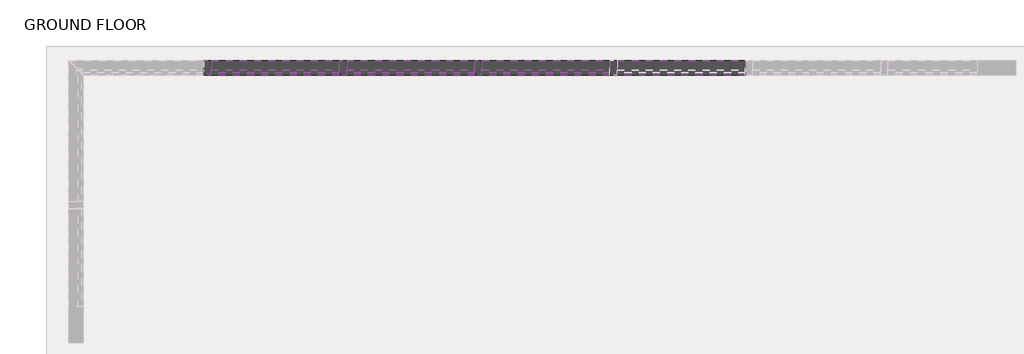
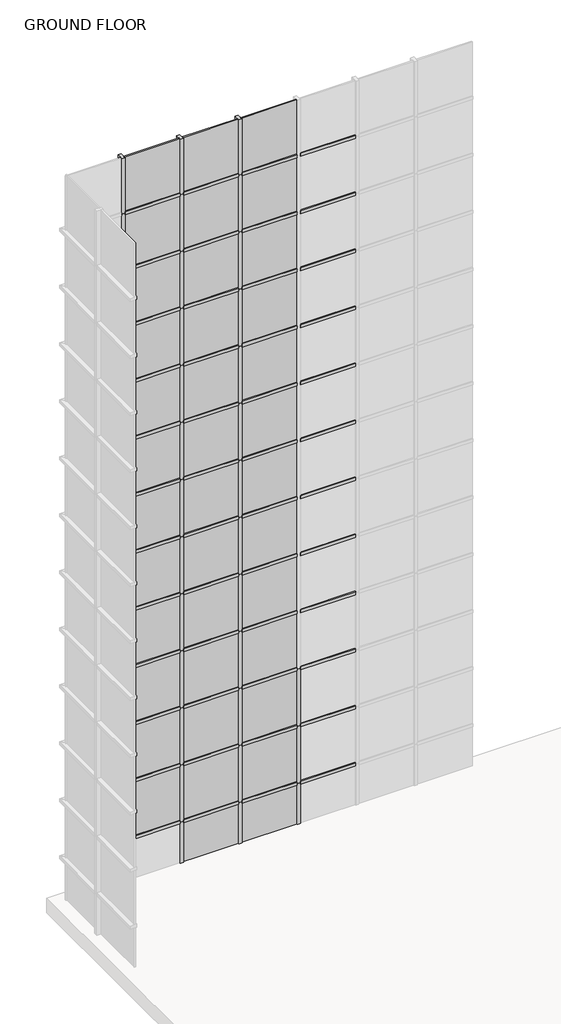
# One storey, part 9 of 16: 90 members, 38 plates.
"""IFC4 building model written with IfcOpenShell, lengths in millimetres."""

from ifc_helpers import new_model, si_unit, origin, place, context, project, spatial, transform, mapped, element, save
from components import member_d518c94e, member_b860638c, member_31fee25f, system_panel_glazed_5cba32e5

model = new_model("IFC4")

# Units and contexts
model_context = context("Model", 3, world=origin())
ifc_project = project(units=[si_unit("LENGTHUNIT", "METRE", prefix="MILLI")], contexts=[model_context])

# Site, building, storey
site = spatial("IfcSite", under=ifc_project)
building = spatial("IfcBuilding", under=site)
storey = spatial("IfcBuildingStorey", under=building, Name="GROUND FLOOR", Elevation=0.0)

# Members
placement = place(None, origin())
member_shape = member_d518c94e(model_context)
element("IfcMember", 1, ObjectType="Rectangular Mullion : 2.5\" x 5\" rectangular", at=placement, inside=storey, context=model_context, shape_type="MappedRepresentation", body=[
    mapped(member_shape, transform((-4463.0248302, 6370.2261968, 1168.8884615), x_axis=(0.0, 0.0, 1.0), y_axis=(0.0, 1.0, 0.0), z_axis=(-1.0, 0.0, 0.0))),
])
element("IfcMember", 2, ObjectType="Rectangular Mullion : 2.5\" x 5\" rectangular", at=placement, inside=storey, context=model_context, shape_type="MappedRepresentation", body=[
    mapped(member_shape, transform((-5628.494061, 6370.2261968, 1168.8884615), x_axis=(0.0, 0.0, 1.0), y_axis=(0.0, 1.0, 0.0), z_axis=(-1.0, 0.0, 0.0))),
])
element("IfcMember", 3, ObjectType="Rectangular Mullion : 2.5\" x 5\" rectangular", at=placement, inside=storey, context=model_context, shape_type="MappedRepresentation", body=[
    mapped(member_shape, transform((-6793.9632917, 6370.2261968, 1168.8884615), x_axis=(0.0, 0.0, 1.0), y_axis=(0.0, 1.0, 0.0), z_axis=(-1.0, 0.0, 0.0))),
])
element("IfcMember", 4, ObjectType="Rectangular Mullion : 2.5\" x 5\" rectangular", at=placement, inside=storey, context=model_context, shape_type="MappedRepresentation", body=[
    mapped(member_shape, transform((-7959.4325224, 6370.2261968, 1168.8884615), x_axis=(0.0, 0.0, 1.0), y_axis=(0.0, 1.0, 0.0), z_axis=(-1.0, 0.0, 0.0))),
])
element("IfcMember", 5, ObjectType="Rectangular Mullion : 2.5\" x 5\" rectangular", at=placement, inside=storey, context=model_context, shape_type="MappedRepresentation", body=[
    mapped(member_shape, transform((-4463.0248302, 6370.2261968, 2369.5269231), x_axis=(0.0, 0.0, 1.0), y_axis=(0.0, 1.0, 0.0), z_axis=(-1.0, 0.0, 0.0))),
])
element("IfcMember", 6, ObjectType="Rectangular Mullion : 2.5\" x 5\" rectangular", at=placement, inside=storey, context=model_context, shape_type="MappedRepresentation", body=[
    mapped(member_shape, transform((-5628.494061, 6370.2261968, 2369.5269231), x_axis=(0.0, 0.0, 1.0), y_axis=(0.0, 1.0, 0.0), z_axis=(-1.0, 0.0, 0.0))),
])
element("IfcMember", 7, ObjectType="Rectangular Mullion : 2.5\" x 5\" rectangular", at=placement, inside=storey, context=model_context, shape_type="MappedRepresentation", body=[
    mapped(member_shape, transform((-6793.9632917, 6370.2261968, 2369.5269231), x_axis=(0.0, 0.0, 1.0), y_axis=(0.0, 1.0, 0.0), z_axis=(-1.0, 0.0, 0.0))),
])
element("IfcMember", 8, ObjectType="Rectangular Mullion : 2.5\" x 5\" rectangular", at=placement, inside=storey, context=model_context, shape_type="MappedRepresentation", body=[
    mapped(member_shape, transform((-7959.4325224, 6370.2261968, 2369.5269231), x_axis=(0.0, 0.0, 1.0), y_axis=(0.0, 1.0, 0.0), z_axis=(-1.0, 0.0, 0.0))),
])
element("IfcMember", 9, ObjectType="Rectangular Mullion : 2.5\" x 5\" rectangular", at=placement, inside=storey, context=model_context, shape_type="MappedRepresentation", body=[
    mapped(member_shape, transform((-4463.0248302, 6370.2261968, 3570.1653846), x_axis=(0.0, 0.0, 1.0), y_axis=(0.0, 1.0, 0.0), z_axis=(-1.0, 0.0, 0.0))),
])
element("IfcMember", 10, ObjectType="Rectangular Mullion : 2.5\" x 5\" rectangular", at=placement, inside=storey, context=model_context, shape_type="MappedRepresentation", body=[
    mapped(member_shape, transform((-5628.494061, 6370.2261968, 3570.1653846), x_axis=(0.0, 0.0, 1.0), y_axis=(0.0, 1.0, 0.0), z_axis=(-1.0, 0.0, 0.0))),
])
element("IfcMember", 11, ObjectType="Rectangular Mullion : 2.5\" x 5\" rectangular", at=placement, inside=storey, context=model_context, shape_type="MappedRepresentation", body=[
    mapped(member_shape, transform((-6793.9632917, 6370.2261968, 3570.1653846), x_axis=(0.0, 0.0, 1.0), y_axis=(0.0, 1.0, 0.0), z_axis=(-1.0, 0.0, 0.0))),
])
element("IfcMember", 12, ObjectType="Rectangular Mullion : 2.5\" x 5\" rectangular", at=placement, inside=storey, context=model_context, shape_type="MappedRepresentation", body=[
    mapped(member_shape, transform((-7959.4325224, 6370.2261968, 3570.1653846), x_axis=(0.0, 0.0, 1.0), y_axis=(0.0, 1.0, 0.0), z_axis=(-1.0, 0.0, 0.0))),
])
element("IfcMember", 13, ObjectType="Rectangular Mullion : 2.5\" x 5\" rectangular", at=placement, inside=storey, context=model_context, shape_type="MappedRepresentation", body=[
    mapped(member_shape, transform((-4463.0248302, 6370.2261968, 4770.8038462), x_axis=(0.0, 0.0, 1.0), y_axis=(0.0, 1.0, 0.0), z_axis=(-1.0, 0.0, 0.0))),
])
element("IfcMember", 14, ObjectType="Rectangular Mullion : 2.5\" x 5\" rectangular", at=placement, inside=storey, context=model_context, shape_type="MappedRepresentation", body=[
    mapped(member_shape, transform((-5628.494061, 6370.2261968, 4770.8038462), x_axis=(0.0, 0.0, 1.0), y_axis=(0.0, 1.0, 0.0), z_axis=(-1.0, 0.0, 0.0))),
])
element("IfcMember", 15, ObjectType="Rectangular Mullion : 2.5\" x 5\" rectangular", at=placement, inside=storey, context=model_context, shape_type="MappedRepresentation", body=[
    mapped(member_shape, transform((-6793.9632917, 6370.2261968, 4770.8038462), x_axis=(0.0, 0.0, 1.0), y_axis=(0.0, 1.0, 0.0), z_axis=(-1.0, 0.0, 0.0))),
])
element("IfcMember", 16, ObjectType="Rectangular Mullion : 2.5\" x 5\" rectangular", at=placement, inside=storey, context=model_context, shape_type="MappedRepresentation", body=[
    mapped(member_shape, transform((-7959.4325224, 6370.2261968, 4770.8038462), x_axis=(0.0, 0.0, 1.0), y_axis=(0.0, 1.0, 0.0), z_axis=(-1.0, 0.0, 0.0))),
])
element("IfcMember", 17, ObjectType="Rectangular Mullion : 2.5\" x 5\" rectangular", at=placement, inside=storey, context=model_context, shape_type="MappedRepresentation", body=[
    mapped(member_shape, transform((-4463.0248302, 6370.2261968, 5971.4423077), x_axis=(0.0, 0.0, 1.0), y_axis=(0.0, 1.0, 0.0), z_axis=(-1.0, 0.0, 0.0))),
])
element("IfcMember", 18, ObjectType="Rectangular Mullion : 2.5\" x 5\" rectangular", at=placement, inside=storey, context=model_context, shape_type="MappedRepresentation", body=[
    mapped(member_shape, transform((-5628.494061, 6370.2261968, 5971.4423077), x_axis=(0.0, 0.0, 1.0), y_axis=(0.0, 1.0, 0.0), z_axis=(-1.0, 0.0, 0.0))),
])
element("IfcMember", 19, ObjectType="Rectangular Mullion : 2.5\" x 5\" rectangular", at=placement, inside=storey, context=model_context, shape_type="MappedRepresentation", body=[
    mapped(member_shape, transform((-6793.9632917, 6370.2261968, 5971.4423077), x_axis=(0.0, 0.0, 1.0), y_axis=(0.0, 1.0, 0.0), z_axis=(-1.0, 0.0, 0.0))),
])
element("IfcMember", 20, ObjectType="Rectangular Mullion : 2.5\" x 5\" rectangular", at=placement, inside=storey, context=model_context, shape_type="MappedRepresentation", body=[
    mapped(member_shape, transform((-7959.4325224, 6370.2261968, 5971.4423077), x_axis=(0.0, 0.0, 1.0), y_axis=(0.0, 1.0, 0.0), z_axis=(-1.0, 0.0, 0.0))),
])
element("IfcMember", 21, ObjectType="Rectangular Mullion : 2.5\" x 5\" rectangular", at=placement, inside=storey, context=model_context, shape_type="MappedRepresentation", body=[
    mapped(member_shape, transform((-4463.0248302, 6370.2261968, 7172.0807692), x_axis=(0.0, 0.0, 1.0), y_axis=(0.0, 1.0, 0.0), z_axis=(-1.0, 0.0, 0.0))),
])
element("IfcMember", 22, ObjectType="Rectangular Mullion : 2.5\" x 5\" rectangular", at=placement, inside=storey, context=model_context, shape_type="MappedRepresentation", body=[
    mapped(member_shape, transform((-5628.494061, 6370.2261968, 7172.0807692), x_axis=(0.0, 0.0, 1.0), y_axis=(0.0, 1.0, 0.0), z_axis=(-1.0, 0.0, 0.0))),
])
element("IfcMember", 23, ObjectType="Rectangular Mullion : 2.5\" x 5\" rectangular", at=placement, inside=storey, context=model_context, shape_type="MappedRepresentation", body=[
    mapped(member_shape, transform((-6793.9632917, 6370.2261968, 7172.0807692), x_axis=(0.0, 0.0, 1.0), y_axis=(0.0, 1.0, 0.0), z_axis=(-1.0, 0.0, 0.0))),
])
element("IfcMember", 24, ObjectType="Rectangular Mullion : 2.5\" x 5\" rectangular", at=placement, inside=storey, context=model_context, shape_type="MappedRepresentation", body=[
    mapped(member_shape, transform((-7959.4325224, 6370.2261968, 7172.0807692), x_axis=(0.0, 0.0, 1.0), y_axis=(0.0, 1.0, 0.0), z_axis=(-1.0, 0.0, 0.0))),
])
element("IfcMember", 25, ObjectType="Rectangular Mullion : 2.5\" x 5\" rectangular", at=placement, inside=storey, context=model_context, shape_type="MappedRepresentation", body=[
    mapped(member_shape, transform((-4463.0248302, 6370.2261968, 8372.7192308), x_axis=(0.0, 0.0, 1.0), y_axis=(0.0, 1.0, 0.0), z_axis=(-1.0, 0.0, 0.0))),
])
element("IfcMember", 26, ObjectType="Rectangular Mullion : 2.5\" x 5\" rectangular", at=placement, inside=storey, context=model_context, shape_type="MappedRepresentation", body=[
    mapped(member_shape, transform((-5628.494061, 6370.2261968, 8372.7192308), x_axis=(0.0, 0.0, 1.0), y_axis=(0.0, 1.0, 0.0), z_axis=(-1.0, 0.0, 0.0))),
])
element("IfcMember", 27, ObjectType="Rectangular Mullion : 2.5\" x 5\" rectangular", at=placement, inside=storey, context=model_context, shape_type="MappedRepresentation", body=[
    mapped(member_shape, transform((-6793.9632917, 6370.2261968, 8372.7192308), x_axis=(0.0, 0.0, 1.0), y_axis=(0.0, 1.0, 0.0), z_axis=(-1.0, 0.0, 0.0))),
])
element("IfcMember", 28, ObjectType="Rectangular Mullion : 2.5\" x 5\" rectangular", at=placement, inside=storey, context=model_context, shape_type="MappedRepresentation", body=[
    mapped(member_shape, transform((-7959.4325224, 6370.2261968, 8372.7192308), x_axis=(0.0, 0.0, 1.0), y_axis=(0.0, 1.0, 0.0), z_axis=(-1.0, 0.0, 0.0))),
])
element("IfcMember", 29, ObjectType="Rectangular Mullion : 2.5\" x 5\" rectangular", at=placement, inside=storey, context=model_context, shape_type="MappedRepresentation", body=[
    mapped(member_shape, transform((-4463.0248302, 6370.2261968, 9573.3576923), x_axis=(0.0, 0.0, 1.0), y_axis=(0.0, 1.0, 0.0), z_axis=(-1.0, 0.0, 0.0))),
])
element("IfcMember", 30, ObjectType="Rectangular Mullion : 2.5\" x 5\" rectangular", at=placement, inside=storey, context=model_context, shape_type="MappedRepresentation", body=[
    mapped(member_shape, transform((-5628.494061, 6370.2261968, 9573.3576923), x_axis=(0.0, 0.0, 1.0), y_axis=(0.0, 1.0, 0.0), z_axis=(-1.0, 0.0, 0.0))),
])
element("IfcMember", 31, ObjectType="Rectangular Mullion : 2.5\" x 5\" rectangular", at=placement, inside=storey, context=model_context, shape_type="MappedRepresentation", body=[
    mapped(member_shape, transform((-6793.9632917, 6370.2261968, 9573.3576923), x_axis=(0.0, 0.0, 1.0), y_axis=(0.0, 1.0, 0.0), z_axis=(-1.0, 0.0, 0.0))),
])
element("IfcMember", 32, ObjectType="Rectangular Mullion : 2.5\" x 5\" rectangular", at=placement, inside=storey, context=model_context, shape_type="MappedRepresentation", body=[
    mapped(member_shape, transform((-7959.4325224, 6370.2261968, 9573.3576923), x_axis=(0.0, 0.0, 1.0), y_axis=(0.0, 1.0, 0.0), z_axis=(-1.0, 0.0, 0.0))),
])
element("IfcMember", 33, ObjectType="Rectangular Mullion : 2.5\" x 5\" rectangular", at=placement, inside=storey, context=model_context, shape_type="MappedRepresentation", body=[
    mapped(member_shape, transform((-4463.0248302, 6370.2261968, 10773.9961538), x_axis=(0.0, 0.0, 1.0), y_axis=(0.0, 1.0, 0.0), z_axis=(-1.0, 0.0, 0.0))),
])
element("IfcMember", 34, ObjectType="Rectangular Mullion : 2.5\" x 5\" rectangular", at=placement, inside=storey, context=model_context, shape_type="MappedRepresentation", body=[
    mapped(member_shape, transform((-5628.494061, 6370.2261968, 10773.9961538), x_axis=(0.0, 0.0, 1.0), y_axis=(0.0, 1.0, 0.0), z_axis=(-1.0, 0.0, 0.0))),
])
element("IfcMember", 35, ObjectType="Rectangular Mullion : 2.5\" x 5\" rectangular", at=placement, inside=storey, context=model_context, shape_type="MappedRepresentation", body=[
    mapped(member_shape, transform((-6793.9632917, 6370.2261968, 10773.9961538), x_axis=(0.0, 0.0, 1.0), y_axis=(0.0, 1.0, 0.0), z_axis=(-1.0, 0.0, 0.0))),
])
element("IfcMember", 36, ObjectType="Rectangular Mullion : 2.5\" x 5\" rectangular", at=placement, inside=storey, context=model_context, shape_type="MappedRepresentation", body=[
    mapped(member_shape, transform((-7959.4325224, 6370.2261968, 10773.9961538), x_axis=(0.0, 0.0, 1.0), y_axis=(0.0, 1.0, 0.0), z_axis=(-1.0, 0.0, 0.0))),
])
element("IfcMember", 37, ObjectType="Rectangular Mullion : 2.5\" x 5\" rectangular", at=placement, inside=storey, context=model_context, shape_type="MappedRepresentation", body=[
    mapped(member_shape, transform((-4463.0248302, 6370.2261968, 11974.6346154), x_axis=(0.0, 0.0, 1.0), y_axis=(0.0, 1.0, 0.0), z_axis=(-1.0, 0.0, 0.0))),
])
element("IfcMember", 38, ObjectType="Rectangular Mullion : 2.5\" x 5\" rectangular", at=placement, inside=storey, context=model_context, shape_type="MappedRepresentation", body=[
    mapped(member_shape, transform((-5628.494061, 6370.2261968, 11974.6346154), x_axis=(0.0, 0.0, 1.0), y_axis=(0.0, 1.0, 0.0), z_axis=(-1.0, 0.0, 0.0))),
])
element("IfcMember", 39, ObjectType="Rectangular Mullion : 2.5\" x 5\" rectangular", at=placement, inside=storey, context=model_context, shape_type="MappedRepresentation", body=[
    mapped(member_shape, transform((-6793.9632917, 6370.2261968, 11974.6346154), x_axis=(0.0, 0.0, 1.0), y_axis=(0.0, 1.0, 0.0), z_axis=(-1.0, 0.0, 0.0))),
])
element("IfcMember", 40, ObjectType="Rectangular Mullion : 2.5\" x 5\" rectangular", at=placement, inside=storey, context=model_context, shape_type="MappedRepresentation", body=[
    mapped(member_shape, transform((-7959.4325224, 6370.2261968, 11974.6346154), x_axis=(0.0, 0.0, 1.0), y_axis=(0.0, 1.0, 0.0), z_axis=(-1.0, 0.0, 0.0))),
])
element("IfcMember", 41, ObjectType="Rectangular Mullion : 2.5\" x 5\" rectangular", at=placement, inside=storey, context=model_context, shape_type="MappedRepresentation", body=[
    mapped(member_shape, transform((-4463.0248302, 6370.2261968, 13175.2730769), x_axis=(0.0, 0.0, 1.0), y_axis=(0.0, 1.0, 0.0), z_axis=(-1.0, 0.0, 0.0))),
])
element("IfcMember", 42, ObjectType="Rectangular Mullion : 2.5\" x 5\" rectangular", at=placement, inside=storey, context=model_context, shape_type="MappedRepresentation", body=[
    mapped(member_shape, transform((-5628.494061, 6370.2261968, 13175.2730769), x_axis=(0.0, 0.0, 1.0), y_axis=(0.0, 1.0, 0.0), z_axis=(-1.0, 0.0, 0.0))),
])
element("IfcMember", 43, ObjectType="Rectangular Mullion : 2.5\" x 5\" rectangular", at=placement, inside=storey, context=model_context, shape_type="MappedRepresentation", body=[
    mapped(member_shape, transform((-6793.9632917, 6370.2261968, 13175.2730769), x_axis=(0.0, 0.0, 1.0), y_axis=(0.0, 1.0, 0.0), z_axis=(-1.0, 0.0, 0.0))),
])
element("IfcMember", 44, ObjectType="Rectangular Mullion : 2.5\" x 5\" rectangular", at=placement, inside=storey, context=model_context, shape_type="MappedRepresentation", body=[
    mapped(member_shape, transform((-7959.4325224, 6370.2261968, 13175.2730769), x_axis=(0.0, 0.0, 1.0), y_axis=(0.0, 1.0, 0.0), z_axis=(-1.0, 0.0, 0.0))),
])
element("IfcMember", 45, ObjectType="Rectangular Mullion : 2.5\" x 5\" rectangular", at=placement, inside=storey, context=model_context, shape_type="MappedRepresentation", body=[
    mapped(member_shape, transform((-4463.0248302, 6370.2261968, 14375.9115385), x_axis=(0.0, 0.0, 1.0), y_axis=(0.0, 1.0, 0.0), z_axis=(-1.0, 0.0, 0.0))),
])
element("IfcMember", 46, ObjectType="Rectangular Mullion : 2.5\" x 5\" rectangular", at=placement, inside=storey, context=model_context, shape_type="MappedRepresentation", body=[
    mapped(member_shape, transform((-5628.494061, 6370.2261968, 14375.9115385), x_axis=(0.0, 0.0, 1.0), y_axis=(0.0, 1.0, 0.0), z_axis=(-1.0, 0.0, 0.0))),
])
element("IfcMember", 47, ObjectType="Rectangular Mullion : 2.5\" x 5\" rectangular", at=placement, inside=storey, context=model_context, shape_type="MappedRepresentation", body=[
    mapped(member_shape, transform((-6793.9632917, 6370.2261968, 14375.9115385), x_axis=(0.0, 0.0, 1.0), y_axis=(0.0, 1.0, 0.0), z_axis=(-1.0, 0.0, 0.0))),
])
element("IfcMember", 48, ObjectType="Rectangular Mullion : 2.5\" x 5\" rectangular", at=placement, inside=storey, context=model_context, shape_type="MappedRepresentation", body=[
    mapped(member_shape, transform((-7959.4325224, 6370.2261968, 14375.9115385), x_axis=(0.0, 0.0, 1.0), y_axis=(0.0, 1.0, 0.0), z_axis=(-1.0, 0.0, 0.0))),
])
member_2_shape = member_b860638c(model_context)
element("IfcMember", 49, ObjectType="Rectangular Mullion : 2.5\" x 5\" rectangular", at=placement, inside=storey, context=model_context, shape_type="MappedRepresentation", body=[
    mapped(member_2_shape, transform((-4494.7748302, 6370.2261968, 0.0), x_axis=(-1.0, 0.0, 0.0), y_axis=(0.0, 1.0, 0.0), z_axis=(0.0, 0.0, -1.0))),
])
element("IfcMember", 50, ObjectType="Rectangular Mullion : 2.5\" x 5\" rectangular", at=placement, inside=storey, context=model_context, shape_type="MappedRepresentation", body=[
    mapped(member_2_shape, transform((-5660.244061, 6370.2261968, 0.0), x_axis=(-1.0, 0.0, 0.0), y_axis=(0.0, 1.0, 0.0), z_axis=(0.0, 0.0, -1.0))),
])
element("IfcMember", 51, ObjectType="Rectangular Mullion : 2.5\" x 5\" rectangular", at=placement, inside=storey, context=model_context, shape_type="MappedRepresentation", body=[
    mapped(member_2_shape, transform((-6825.7132917, 6370.2261968, 0.0), x_axis=(-1.0, 0.0, 0.0), y_axis=(0.0, 1.0, 0.0), z_axis=(0.0, 0.0, -1.0))),
])
element("IfcMember", 52, ObjectType="Rectangular Mullion : 2.5\" x 5\" rectangular", at=placement, inside=storey, context=model_context, shape_type="MappedRepresentation", body=[
    mapped(member_2_shape, transform((-7991.1825224, 6370.2261968, 0.0), x_axis=(-1.0, 0.0, 0.0), y_axis=(0.0, 1.0, 0.0), z_axis=(0.0, 0.0, -1.0))),
])
member_3_shape = member_31fee25f(model_context)
element("IfcMember", 53, ObjectType="Rectangular Mullion : 2.5\" x 5\" rectangular", at=placement, inside=storey, context=model_context, shape_type="MappedRepresentation", body=[
    mapped(member_3_shape, transform((-4494.7748302, 6370.2261968, 1168.8884615), x_axis=(-1.0, 0.0, 0.0), y_axis=(0.0, 1.0, 0.0), z_axis=(0.0, 0.0, -1.0))),
])
element("IfcMember", 54, ObjectType="Rectangular Mullion : 2.5\" x 5\" rectangular", at=placement, inside=storey, context=model_context, shape_type="MappedRepresentation", body=[
    mapped(member_3_shape, transform((-5660.244061, 6370.2261968, 1168.8884615), x_axis=(-1.0, 0.0, 0.0), y_axis=(0.0, 1.0, 0.0), z_axis=(0.0, 0.0, -1.0))),
])
element("IfcMember", 55, ObjectType="Rectangular Mullion : 2.5\" x 5\" rectangular", at=placement, inside=storey, context=model_context, shape_type="MappedRepresentation", body=[
    mapped(member_3_shape, transform((-6825.7132917, 6370.2261968, 1168.8884615), x_axis=(-1.0, 0.0, 0.0), y_axis=(0.0, 1.0, 0.0), z_axis=(0.0, 0.0, -1.0))),
])
element("IfcMember", 56, ObjectType="Rectangular Mullion : 2.5\" x 5\" rectangular", at=placement, inside=storey, context=model_context, shape_type="MappedRepresentation", body=[
    mapped(member_3_shape, transform((-7991.1825224, 6370.2261968, 1168.8884615), x_axis=(-1.0, 0.0, 0.0), y_axis=(0.0, 1.0, 0.0), z_axis=(0.0, 0.0, -1.0))),
])
element("IfcMember", 57, ObjectType="Rectangular Mullion : 2.5\" x 5\" rectangular", at=placement, inside=storey, context=model_context, shape_type="MappedRepresentation", body=[
    mapped(member_3_shape, transform((-4494.7748302, 6370.2261968, 2369.5269231), x_axis=(-1.0, 0.0, 0.0), y_axis=(0.0, 1.0, 0.0), z_axis=(0.0, 0.0, -1.0))),
])
element("IfcMember", 58, ObjectType="Rectangular Mullion : 2.5\" x 5\" rectangular", at=placement, inside=storey, context=model_context, shape_type="MappedRepresentation", body=[
    mapped(member_3_shape, transform((-5660.244061, 6370.2261968, 2369.5269231), x_axis=(-1.0, 0.0, 0.0), y_axis=(0.0, 1.0, 0.0), z_axis=(0.0, 0.0, -1.0))),
])
element("IfcMember", 59, ObjectType="Rectangular Mullion : 2.5\" x 5\" rectangular", at=placement, inside=storey, context=model_context, shape_type="MappedRepresentation", body=[
    mapped(member_3_shape, transform((-6825.7132917, 6370.2261968, 2369.5269231), x_axis=(-1.0, 0.0, 0.0), y_axis=(0.0, 1.0, 0.0), z_axis=(0.0, 0.0, -1.0))),
])
element("IfcMember", 60, ObjectType="Rectangular Mullion : 2.5\" x 5\" rectangular", at=placement, inside=storey, context=model_context, shape_type="MappedRepresentation", body=[
    mapped(member_3_shape, transform((-7991.1825224, 6370.2261968, 2369.5269231), x_axis=(-1.0, 0.0, 0.0), y_axis=(0.0, 1.0, 0.0), z_axis=(0.0, 0.0, -1.0))),
])
element("IfcMember", 61, ObjectType="Rectangular Mullion : 2.5\" x 5\" rectangular", at=placement, inside=storey, context=model_context, shape_type="MappedRepresentation", body=[
    mapped(member_3_shape, transform((-5660.244061, 6370.2261968, 3570.1653846), x_axis=(-1.0, 0.0, 0.0), y_axis=(0.0, 1.0, 0.0), z_axis=(0.0, 0.0, -1.0))),
])
element("IfcMember", 62, ObjectType="Rectangular Mullion : 2.5\" x 5\" rectangular", at=placement, inside=storey, context=model_context, shape_type="MappedRepresentation", body=[
    mapped(member_3_shape, transform((-6825.7132917, 6370.2261968, 3570.1653846), x_axis=(-1.0, 0.0, 0.0), y_axis=(0.0, 1.0, 0.0), z_axis=(0.0, 0.0, -1.0))),
])
element("IfcMember", 63, ObjectType="Rectangular Mullion : 2.5\" x 5\" rectangular", at=placement, inside=storey, context=model_context, shape_type="MappedRepresentation", body=[
    mapped(member_3_shape, transform((-7991.1825224, 6370.2261968, 3570.1653846), x_axis=(-1.0, 0.0, 0.0), y_axis=(0.0, 1.0, 0.0), z_axis=(0.0, 0.0, -1.0))),
])
element("IfcMember", 64, ObjectType="Rectangular Mullion : 2.5\" x 5\" rectangular", at=placement, inside=storey, context=model_context, shape_type="MappedRepresentation", body=[
    mapped(member_3_shape, transform((-5660.244061, 6370.2261968, 4770.8038462), x_axis=(-1.0, 0.0, 0.0), y_axis=(0.0, 1.0, 0.0), z_axis=(0.0, 0.0, -1.0))),
])
element("IfcMember", 65, ObjectType="Rectangular Mullion : 2.5\" x 5\" rectangular", at=placement, inside=storey, context=model_context, shape_type="MappedRepresentation", body=[
    mapped(member_3_shape, transform((-6825.7132917, 6370.2261968, 4770.8038462), x_axis=(-1.0, 0.0, 0.0), y_axis=(0.0, 1.0, 0.0), z_axis=(0.0, 0.0, -1.0))),
])
element("IfcMember", 66, ObjectType="Rectangular Mullion : 2.5\" x 5\" rectangular", at=placement, inside=storey, context=model_context, shape_type="MappedRepresentation", body=[
    mapped(member_3_shape, transform((-7991.1825224, 6370.2261968, 4770.8038462), x_axis=(-1.0, 0.0, 0.0), y_axis=(0.0, 1.0, 0.0), z_axis=(0.0, 0.0, -1.0))),
])
element("IfcMember", 67, ObjectType="Rectangular Mullion : 2.5\" x 5\" rectangular", at=placement, inside=storey, context=model_context, shape_type="MappedRepresentation", body=[
    mapped(member_3_shape, transform((-5660.244061, 6370.2261968, 5971.4423077), x_axis=(-1.0, 0.0, 0.0), y_axis=(0.0, 1.0, 0.0), z_axis=(0.0, 0.0, -1.0))),
])
element("IfcMember", 68, ObjectType="Rectangular Mullion : 2.5\" x 5\" rectangular", at=placement, inside=storey, context=model_context, shape_type="MappedRepresentation", body=[
    mapped(member_3_shape, transform((-6825.7132917, 6370.2261968, 5971.4423077), x_axis=(-1.0, 0.0, 0.0), y_axis=(0.0, 1.0, 0.0), z_axis=(0.0, 0.0, -1.0))),
])
element("IfcMember", 69, ObjectType="Rectangular Mullion : 2.5\" x 5\" rectangular", at=placement, inside=storey, context=model_context, shape_type="MappedRepresentation", body=[
    mapped(member_3_shape, transform((-7991.1825224, 6370.2261968, 5971.4423077), x_axis=(-1.0, 0.0, 0.0), y_axis=(0.0, 1.0, 0.0), z_axis=(0.0, 0.0, -1.0))),
])
element("IfcMember", 70, ObjectType="Rectangular Mullion : 2.5\" x 5\" rectangular", at=placement, inside=storey, context=model_context, shape_type="MappedRepresentation", body=[
    mapped(member_3_shape, transform((-5660.244061, 6370.2261968, 7172.0807692), x_axis=(-1.0, 0.0, 0.0), y_axis=(0.0, 1.0, 0.0), z_axis=(0.0, 0.0, -1.0))),
])
element("IfcMember", 71, ObjectType="Rectangular Mullion : 2.5\" x 5\" rectangular", at=placement, inside=storey, context=model_context, shape_type="MappedRepresentation", body=[
    mapped(member_3_shape, transform((-6825.7132917, 6370.2261968, 7172.0807692), x_axis=(-1.0, 0.0, 0.0), y_axis=(0.0, 1.0, 0.0), z_axis=(0.0, 0.0, -1.0))),
])
element("IfcMember", 72, ObjectType="Rectangular Mullion : 2.5\" x 5\" rectangular", at=placement, inside=storey, context=model_context, shape_type="MappedRepresentation", body=[
    mapped(member_3_shape, transform((-7991.1825224, 6370.2261968, 7172.0807692), x_axis=(-1.0, 0.0, 0.0), y_axis=(0.0, 1.0, 0.0), z_axis=(0.0, 0.0, -1.0))),
])
element("IfcMember", 73, ObjectType="Rectangular Mullion : 2.5\" x 5\" rectangular", at=placement, inside=storey, context=model_context, shape_type="MappedRepresentation", body=[
    mapped(member_3_shape, transform((-5660.244061, 6370.2261968, 8372.7192308), x_axis=(-1.0, 0.0, 0.0), y_axis=(0.0, 1.0, 0.0), z_axis=(0.0, 0.0, -1.0))),
])
element("IfcMember", 74, ObjectType="Rectangular Mullion : 2.5\" x 5\" rectangular", at=placement, inside=storey, context=model_context, shape_type="MappedRepresentation", body=[
    mapped(member_3_shape, transform((-6825.7132917, 6370.2261968, 8372.7192308), x_axis=(-1.0, 0.0, 0.0), y_axis=(0.0, 1.0, 0.0), z_axis=(0.0, 0.0, -1.0))),
])
element("IfcMember", 75, ObjectType="Rectangular Mullion : 2.5\" x 5\" rectangular", at=placement, inside=storey, context=model_context, shape_type="MappedRepresentation", body=[
    mapped(member_3_shape, transform((-7991.1825224, 6370.2261968, 8372.7192308), x_axis=(-1.0, 0.0, 0.0), y_axis=(0.0, 1.0, 0.0), z_axis=(0.0, 0.0, -1.0))),
])
element("IfcMember", 76, ObjectType="Rectangular Mullion : 2.5\" x 5\" rectangular", at=placement, inside=storey, context=model_context, shape_type="MappedRepresentation", body=[
    mapped(member_3_shape, transform((-5660.244061, 6370.2261968, 9573.3576923), x_axis=(-1.0, 0.0, 0.0), y_axis=(0.0, 1.0, 0.0), z_axis=(0.0, 0.0, -1.0))),
])
element("IfcMember", 77, ObjectType="Rectangular Mullion : 2.5\" x 5\" rectangular", at=placement, inside=storey, context=model_context, shape_type="MappedRepresentation", body=[
    mapped(member_3_shape, transform((-6825.7132917, 6370.2261968, 9573.3576923), x_axis=(-1.0, 0.0, 0.0), y_axis=(0.0, 1.0, 0.0), z_axis=(0.0, 0.0, -1.0))),
])
element("IfcMember", 78, ObjectType="Rectangular Mullion : 2.5\" x 5\" rectangular", at=placement, inside=storey, context=model_context, shape_type="MappedRepresentation", body=[
    mapped(member_3_shape, transform((-7991.1825224, 6370.2261968, 9573.3576923), x_axis=(-1.0, 0.0, 0.0), y_axis=(0.0, 1.0, 0.0), z_axis=(0.0, 0.0, -1.0))),
])
element("IfcMember", 79, ObjectType="Rectangular Mullion : 2.5\" x 5\" rectangular", at=placement, inside=storey, context=model_context, shape_type="MappedRepresentation", body=[
    mapped(member_3_shape, transform((-5660.244061, 6370.2261968, 10773.9961538), x_axis=(-1.0, 0.0, 0.0), y_axis=(0.0, 1.0, 0.0), z_axis=(0.0, 0.0, -1.0))),
])
element("IfcMember", 80, ObjectType="Rectangular Mullion : 2.5\" x 5\" rectangular", at=placement, inside=storey, context=model_context, shape_type="MappedRepresentation", body=[
    mapped(member_3_shape, transform((-6825.7132917, 6370.2261968, 10773.9961538), x_axis=(-1.0, 0.0, 0.0), y_axis=(0.0, 1.0, 0.0), z_axis=(0.0, 0.0, -1.0))),
])
element("IfcMember", 81, ObjectType="Rectangular Mullion : 2.5\" x 5\" rectangular", at=placement, inside=storey, context=model_context, shape_type="MappedRepresentation", body=[
    mapped(member_3_shape, transform((-7991.1825224, 6370.2261968, 10773.9961538), x_axis=(-1.0, 0.0, 0.0), y_axis=(0.0, 1.0, 0.0), z_axis=(0.0, 0.0, -1.0))),
])
element("IfcMember", 82, ObjectType="Rectangular Mullion : 2.5\" x 5\" rectangular", at=placement, inside=storey, context=model_context, shape_type="MappedRepresentation", body=[
    mapped(member_3_shape, transform((-5660.244061, 6370.2261968, 11974.6346154), x_axis=(-1.0, 0.0, 0.0), y_axis=(0.0, 1.0, 0.0), z_axis=(0.0, 0.0, -1.0))),
])
element("IfcMember", 83, ObjectType="Rectangular Mullion : 2.5\" x 5\" rectangular", at=placement, inside=storey, context=model_context, shape_type="MappedRepresentation", body=[
    mapped(member_3_shape, transform((-6825.7132917, 6370.2261968, 11974.6346154), x_axis=(-1.0, 0.0, 0.0), y_axis=(0.0, 1.0, 0.0), z_axis=(0.0, 0.0, -1.0))),
])
element("IfcMember", 84, ObjectType="Rectangular Mullion : 2.5\" x 5\" rectangular", at=placement, inside=storey, context=model_context, shape_type="MappedRepresentation", body=[
    mapped(member_3_shape, transform((-7991.1825224, 6370.2261968, 11974.6346154), x_axis=(-1.0, 0.0, 0.0), y_axis=(0.0, 1.0, 0.0), z_axis=(0.0, 0.0, -1.0))),
])
element("IfcMember", 85, ObjectType="Rectangular Mullion : 2.5\" x 5\" rectangular", at=placement, inside=storey, context=model_context, shape_type="MappedRepresentation", body=[
    mapped(member_3_shape, transform((-5660.244061, 6370.2261968, 13175.2730769), x_axis=(-1.0, 0.0, 0.0), y_axis=(0.0, 1.0, 0.0), z_axis=(0.0, 0.0, -1.0))),
])
element("IfcMember", 86, ObjectType="Rectangular Mullion : 2.5\" x 5\" rectangular", at=placement, inside=storey, context=model_context, shape_type="MappedRepresentation", body=[
    mapped(member_3_shape, transform((-6825.7132917, 6370.2261968, 13175.2730769), x_axis=(-1.0, 0.0, 0.0), y_axis=(0.0, 1.0, 0.0), z_axis=(0.0, 0.0, -1.0))),
])
element("IfcMember", 87, ObjectType="Rectangular Mullion : 2.5\" x 5\" rectangular", at=placement, inside=storey, context=model_context, shape_type="MappedRepresentation", body=[
    mapped(member_3_shape, transform((-7991.1825224, 6370.2261968, 13175.2730769), x_axis=(-1.0, 0.0, 0.0), y_axis=(0.0, 1.0, 0.0), z_axis=(0.0, 0.0, -1.0))),
])
element("IfcMember", 88, ObjectType="Rectangular Mullion : 2.5\" x 5\" rectangular", at=placement, inside=storey, context=model_context, shape_type="MappedRepresentation", body=[
    mapped(member_2_shape, transform((-5660.244061, 6370.2261968, 14375.9115385), x_axis=(-1.0, 0.0, 0.0), y_axis=(0.0, 1.0, 0.0), z_axis=(0.0, 0.0, -1.0))),
])
element("IfcMember", 89, ObjectType="Rectangular Mullion : 2.5\" x 5\" rectangular", at=placement, inside=storey, context=model_context, shape_type="MappedRepresentation", body=[
    mapped(member_2_shape, transform((-6825.7132917, 6370.2261968, 14375.9115385), x_axis=(-1.0, 0.0, 0.0), y_axis=(0.0, 1.0, 0.0), z_axis=(0.0, 0.0, -1.0))),
])
element("IfcMember", 90, ObjectType="Rectangular Mullion : 2.5\" x 5\" rectangular", at=placement, inside=storey, context=model_context, shape_type="MappedRepresentation", body=[
    mapped(member_2_shape, transform((-7991.1825224, 6370.2261968, 14375.9115385), x_axis=(-1.0, 0.0, 0.0), y_axis=(0.0, 1.0, 0.0), z_axis=(0.0, 0.0, -1.0))),
])

# Plates
system_panel_glazed_shape = system_panel_glazed_5cba32e5(model_context)
element("IfcPlate", 91, ObjectType="System Panel : Glazed", at=placement, inside=storey, context=model_context, shape_type="MappedRepresentation", body=[
    mapped(system_panel_glazed_shape, transform((-5077.5094456, 6370.2261968, 0.0), x_axis=(-1.0, 0.0, 0.0), y_axis=(0.0, -1.0, 0.0), z_axis=(0.0, 0.0, 1.0))),
])
element("IfcPlate", 92, ObjectType="System Panel : Glazed", at=placement, inside=storey, context=model_context, shape_type="MappedRepresentation", body=[
    mapped(system_panel_glazed_shape, transform((-6242.9786763, 6370.2261968, 0.0), x_axis=(-1.0, 0.0, 0.0), y_axis=(0.0, -1.0, 0.0), z_axis=(0.0, 0.0, 1.0))),
])
element("IfcPlate", 93, ObjectType="System Panel : Glazed", at=placement, inside=storey, context=model_context, shape_type="MappedRepresentation", body=[
    mapped(system_panel_glazed_shape, transform((-5077.5094456, 6370.2261968, 1200.6384615), x_axis=(-1.0, 0.0, 0.0), y_axis=(0.0, -1.0, 0.0), z_axis=(0.0, 0.0, 1.0))),
])
element("IfcPlate", 94, ObjectType="System Panel : Glazed", at=placement, inside=storey, context=model_context, shape_type="MappedRepresentation", body=[
    mapped(system_panel_glazed_shape, transform((-6242.9786763, 6370.2261968, 1200.6384615), x_axis=(-1.0, 0.0, 0.0), y_axis=(0.0, -1.0, 0.0), z_axis=(0.0, 0.0, 1.0))),
])
element("IfcPlate", 95, ObjectType="System Panel : Glazed", at=placement, inside=storey, context=model_context, shape_type="MappedRepresentation", body=[
    mapped(system_panel_glazed_shape, transform((-7408.447907, 6370.2261968, 1200.6384615), x_axis=(-1.0, 0.0, 0.0), y_axis=(0.0, -1.0, 0.0), z_axis=(0.0, 0.0, 1.0))),
])
element("IfcPlate", 96, ObjectType="System Panel : Glazed", at=placement, inside=storey, context=model_context, shape_type="MappedRepresentation", body=[
    mapped(system_panel_glazed_shape, transform((-5077.5094456, 6370.2261968, 2401.2769231), x_axis=(-1.0, 0.0, 0.0), y_axis=(0.0, -1.0, 0.0), z_axis=(0.0, 0.0, 1.0))),
])
element("IfcPlate", 97, ObjectType="System Panel : Glazed", at=placement, inside=storey, context=model_context, shape_type="MappedRepresentation", body=[
    mapped(system_panel_glazed_shape, transform((-6242.9786763, 6370.2261968, 2401.2769231), x_axis=(-1.0, 0.0, 0.0), y_axis=(0.0, -1.0, 0.0), z_axis=(0.0, 0.0, 1.0))),
])
element("IfcPlate", 98, ObjectType="System Panel : Glazed", at=placement, inside=storey, context=model_context, shape_type="MappedRepresentation", body=[
    mapped(system_panel_glazed_shape, transform((-7408.447907, 6370.2261968, 2401.2769231), x_axis=(-1.0, 0.0, 0.0), y_axis=(0.0, -1.0, 0.0), z_axis=(0.0, 0.0, 1.0))),
])
element("IfcPlate", 99, ObjectType="System Panel : Glazed", at=placement, inside=storey, context=model_context, shape_type="MappedRepresentation", body=[
    mapped(system_panel_glazed_shape, transform((-5077.5094456, 6370.2261968, 3601.9153846), x_axis=(-1.0, 0.0, 0.0), y_axis=(0.0, -1.0, 0.0), z_axis=(0.0, 0.0, 1.0))),
])
element("IfcPlate", 100, ObjectType="System Panel : Glazed", at=placement, inside=storey, context=model_context, shape_type="MappedRepresentation", body=[
    mapped(system_panel_glazed_shape, transform((-6242.9786763, 6370.2261968, 3601.9153846), x_axis=(-1.0, 0.0, 0.0), y_axis=(0.0, -1.0, 0.0), z_axis=(0.0, 0.0, 1.0))),
])
element("IfcPlate", 101, ObjectType="System Panel : Glazed", at=placement, inside=storey, context=model_context, shape_type="MappedRepresentation", body=[
    mapped(system_panel_glazed_shape, transform((-7408.447907, 6370.2261968, 3601.9153846), x_axis=(-1.0, 0.0, 0.0), y_axis=(0.0, -1.0, 0.0), z_axis=(0.0, 0.0, 1.0))),
])
element("IfcPlate", 102, ObjectType="System Panel : Glazed", at=placement, inside=storey, context=model_context, shape_type="MappedRepresentation", body=[
    mapped(system_panel_glazed_shape, transform((-5077.5094456, 6370.2261968, 4802.5538462), x_axis=(-1.0, 0.0, 0.0), y_axis=(0.0, -1.0, 0.0), z_axis=(0.0, 0.0, 1.0))),
])
element("IfcPlate", 103, ObjectType="System Panel : Glazed", at=placement, inside=storey, context=model_context, shape_type="MappedRepresentation", body=[
    mapped(system_panel_glazed_shape, transform((-6242.9786763, 6370.2261968, 4802.5538462), x_axis=(-1.0, 0.0, 0.0), y_axis=(0.0, -1.0, 0.0), z_axis=(0.0, 0.0, 1.0))),
])
element("IfcPlate", 104, ObjectType="System Panel : Glazed", at=placement, inside=storey, context=model_context, shape_type="MappedRepresentation", body=[
    mapped(system_panel_glazed_shape, transform((-7408.447907, 6370.2261968, 4802.5538462), x_axis=(-1.0, 0.0, 0.0), y_axis=(0.0, -1.0, 0.0), z_axis=(0.0, 0.0, 1.0))),
])
element("IfcPlate", 105, ObjectType="System Panel : Glazed", at=placement, inside=storey, context=model_context, shape_type="MappedRepresentation", body=[
    mapped(system_panel_glazed_shape, transform((-5077.5094456, 6370.2261968, 6003.1923077), x_axis=(-1.0, 0.0, 0.0), y_axis=(0.0, -1.0, 0.0), z_axis=(0.0, 0.0, 1.0))),
])
element("IfcPlate", 106, ObjectType="System Panel : Glazed", at=placement, inside=storey, context=model_context, shape_type="MappedRepresentation", body=[
    mapped(system_panel_glazed_shape, transform((-6242.9786763, 6370.2261968, 6003.1923077), x_axis=(-1.0, 0.0, 0.0), y_axis=(0.0, -1.0, 0.0), z_axis=(0.0, 0.0, 1.0))),
])
element("IfcPlate", 107, ObjectType="System Panel : Glazed", at=placement, inside=storey, context=model_context, shape_type="MappedRepresentation", body=[
    mapped(system_panel_glazed_shape, transform((-7408.447907, 6370.2261968, 6003.1923077), x_axis=(-1.0, 0.0, 0.0), y_axis=(0.0, -1.0, 0.0), z_axis=(0.0, 0.0, 1.0))),
])
element("IfcPlate", 108, ObjectType="System Panel : Glazed", at=placement, inside=storey, context=model_context, shape_type="MappedRepresentation", body=[
    mapped(system_panel_glazed_shape, transform((-5077.5094456, 6370.2261968, 7203.8307692), x_axis=(-1.0, 0.0, 0.0), y_axis=(0.0, -1.0, 0.0), z_axis=(0.0, 0.0, 1.0))),
])
element("IfcPlate", 109, ObjectType="System Panel : Glazed", at=placement, inside=storey, context=model_context, shape_type="MappedRepresentation", body=[
    mapped(system_panel_glazed_shape, transform((-6242.9786763, 6370.2261968, 7203.8307692), x_axis=(-1.0, 0.0, 0.0), y_axis=(0.0, -1.0, 0.0), z_axis=(0.0, 0.0, 1.0))),
])
element("IfcPlate", 110, ObjectType="System Panel : Glazed", at=placement, inside=storey, context=model_context, shape_type="MappedRepresentation", body=[
    mapped(system_panel_glazed_shape, transform((-7408.447907, 6370.2261968, 7203.8307692), x_axis=(-1.0, 0.0, 0.0), y_axis=(0.0, -1.0, 0.0), z_axis=(0.0, 0.0, 1.0))),
])
element("IfcPlate", 111, ObjectType="System Panel : Glazed", at=placement, inside=storey, context=model_context, shape_type="MappedRepresentation", body=[
    mapped(system_panel_glazed_shape, transform((-5077.5094456, 6370.2261968, 8404.4692308), x_axis=(-1.0, 0.0, 0.0), y_axis=(0.0, -1.0, 0.0), z_axis=(0.0, 0.0, 1.0))),
])
element("IfcPlate", 112, ObjectType="System Panel : Glazed", at=placement, inside=storey, context=model_context, shape_type="MappedRepresentation", body=[
    mapped(system_panel_glazed_shape, transform((-6242.9786763, 6370.2261968, 8404.4692308), x_axis=(-1.0, 0.0, 0.0), y_axis=(0.0, -1.0, 0.0), z_axis=(0.0, 0.0, 1.0))),
])
element("IfcPlate", 113, ObjectType="System Panel : Glazed", at=placement, inside=storey, context=model_context, shape_type="MappedRepresentation", body=[
    mapped(system_panel_glazed_shape, transform((-7408.447907, 6370.2261968, 8404.4692308), x_axis=(-1.0, 0.0, 0.0), y_axis=(0.0, -1.0, 0.0), z_axis=(0.0, 0.0, 1.0))),
])
element("IfcPlate", 114, ObjectType="System Panel : Glazed", at=placement, inside=storey, context=model_context, shape_type="MappedRepresentation", body=[
    mapped(system_panel_glazed_shape, transform((-5077.5094456, 6370.2261968, 9605.1076923), x_axis=(-1.0, 0.0, 0.0), y_axis=(0.0, -1.0, 0.0), z_axis=(0.0, 0.0, 1.0))),
])
element("IfcPlate", 115, ObjectType="System Panel : Glazed", at=placement, inside=storey, context=model_context, shape_type="MappedRepresentation", body=[
    mapped(system_panel_glazed_shape, transform((-6242.9786763, 6370.2261968, 9605.1076923), x_axis=(-1.0, 0.0, 0.0), y_axis=(0.0, -1.0, 0.0), z_axis=(0.0, 0.0, 1.0))),
])
element("IfcPlate", 116, ObjectType="System Panel : Glazed", at=placement, inside=storey, context=model_context, shape_type="MappedRepresentation", body=[
    mapped(system_panel_glazed_shape, transform((-7408.447907, 6370.2261968, 9605.1076923), x_axis=(-1.0, 0.0, 0.0), y_axis=(0.0, -1.0, 0.0), z_axis=(0.0, 0.0, 1.0))),
])
element("IfcPlate", 117, ObjectType="System Panel : Glazed", at=placement, inside=storey, context=model_context, shape_type="MappedRepresentation", body=[
    mapped(system_panel_glazed_shape, transform((-5077.5094456, 6370.2261968, 10805.7461538), x_axis=(-1.0, 0.0, 0.0), y_axis=(0.0, -1.0, 0.0), z_axis=(0.0, 0.0, 1.0))),
])
element("IfcPlate", 118, ObjectType="System Panel : Glazed", at=placement, inside=storey, context=model_context, shape_type="MappedRepresentation", body=[
    mapped(system_panel_glazed_shape, transform((-6242.9786763, 6370.2261968, 10805.7461538), x_axis=(-1.0, 0.0, 0.0), y_axis=(0.0, -1.0, 0.0), z_axis=(0.0, 0.0, 1.0))),
])
element("IfcPlate", 119, ObjectType="System Panel : Glazed", at=placement, inside=storey, context=model_context, shape_type="MappedRepresentation", body=[
    mapped(system_panel_glazed_shape, transform((-7408.447907, 6370.2261968, 10805.7461538), x_axis=(-1.0, 0.0, 0.0), y_axis=(0.0, -1.0, 0.0), z_axis=(0.0, 0.0, 1.0))),
])
element("IfcPlate", 120, ObjectType="System Panel : Glazed", at=placement, inside=storey, context=model_context, shape_type="MappedRepresentation", body=[
    mapped(system_panel_glazed_shape, transform((-5077.5094456, 6370.2261968, 12006.3846154), x_axis=(-1.0, 0.0, 0.0), y_axis=(0.0, -1.0, 0.0), z_axis=(0.0, 0.0, 1.0))),
])
element("IfcPlate", 121, ObjectType="System Panel : Glazed", at=placement, inside=storey, context=model_context, shape_type="MappedRepresentation", body=[
    mapped(system_panel_glazed_shape, transform((-6242.9786763, 6370.2261968, 12006.3846154), x_axis=(-1.0, 0.0, 0.0), y_axis=(0.0, -1.0, 0.0), z_axis=(0.0, 0.0, 1.0))),
])
element("IfcPlate", 122, ObjectType="System Panel : Glazed", at=placement, inside=storey, context=model_context, shape_type="MappedRepresentation", body=[
    mapped(system_panel_glazed_shape, transform((-7408.447907, 6370.2261968, 12006.3846154), x_axis=(-1.0, 0.0, 0.0), y_axis=(0.0, -1.0, 0.0), z_axis=(0.0, 0.0, 1.0))),
])
element("IfcPlate", 123, ObjectType="System Panel : Glazed", at=placement, inside=storey, context=model_context, shape_type="MappedRepresentation", body=[
    mapped(system_panel_glazed_shape, transform((-5077.5094456, 6370.2261968, 13207.0230769), x_axis=(-1.0, 0.0, 0.0), y_axis=(0.0, -1.0, 0.0), z_axis=(0.0, 0.0, 1.0))),
])
element("IfcPlate", 124, ObjectType="System Panel : Glazed", at=placement, inside=storey, context=model_context, shape_type="MappedRepresentation", body=[
    mapped(system_panel_glazed_shape, transform((-6242.9786763, 6370.2261968, 13207.0230769), x_axis=(-1.0, 0.0, 0.0), y_axis=(0.0, -1.0, 0.0), z_axis=(0.0, 0.0, 1.0))),
])
element("IfcPlate", 125, ObjectType="System Panel : Glazed", at=placement, inside=storey, context=model_context, shape_type="MappedRepresentation", body=[
    mapped(system_panel_glazed_shape, transform((-7408.447907, 6370.2261968, 13207.0230769), x_axis=(-1.0, 0.0, 0.0), y_axis=(0.0, -1.0, 0.0), z_axis=(0.0, 0.0, 1.0))),
])
element("IfcPlate", 126, ObjectType="System Panel : Glazed", at=placement, inside=storey, context=model_context, shape_type="MappedRepresentation", body=[
    mapped(system_panel_glazed_shape, transform((-5077.5094456, 6370.2261968, 14407.6615385), x_axis=(-1.0, 0.0, 0.0), y_axis=(0.0, -1.0, 0.0), z_axis=(0.0, 0.0, 1.0))),
])
element("IfcPlate", 127, ObjectType="System Panel : Glazed", at=placement, inside=storey, context=model_context, shape_type="MappedRepresentation", body=[
    mapped(system_panel_glazed_shape, transform((-6242.9786763, 6370.2261968, 14407.6615385), x_axis=(-1.0, 0.0, 0.0), y_axis=(0.0, -1.0, 0.0), z_axis=(0.0, 0.0, 1.0))),
])
element("IfcPlate", 128, ObjectType="System Panel : Glazed", at=placement, inside=storey, context=model_context, shape_type="MappedRepresentation", body=[
    mapped(system_panel_glazed_shape, transform((-7408.447907, 6370.2261968, 14407.6615385), x_axis=(-1.0, 0.0, 0.0), y_axis=(0.0, -1.0, 0.0), z_axis=(0.0, 0.0, 1.0))),
])

save(model, "model.ifc")

# Revit data of these elements
# Type "Rectangular Mullion : 2.5\" x 5\" rectangular"
#   built-in parameter 1007304 = 0.416667 (stored number, unit not read)
#   built-in parameter 1007301 = 0.104167 (stored number, unit not read)
#   built-in parameter 1007300 = 0.104167 (stored number, unit not read)
# Type "System Panel : Glazed"
#   Construction Type Id = "GSP4R"
#   Analytic Construction = "1/8 in Pilkington single glazing"
#   Visual Light Transmittance = 0.9
#   Solar Heat Gain Coefficient = 0.86
#   Heat Transfer Coefficient (U) = 1.18115 BTU/(h·ft²·°F)
#   Define Thermal Properties by = 1
# Elements 1, 2, 3, 4, 5, 6, 7, 8, 9, 10, 11, 12, 13, 14, 15, 16, 17, 18, 19, 20, 21, 22, 23, 24, 25, 26, 27, 28, 29, 30, 31, 32, 33, 34, 35, 36, 37, 38, 39, 40, 41, 42, 43, 44, 45, 46, 47, 48, 49, 50, 51, 52, 53, 54, 55, 56, 57, 58, 59, 60, 61, 62, 63, 64, 65, 66, 67, 68, 69, 70, 71, 72, 73, 74, 75, 76, 77, 78, 79, 80, 81, 82, 83, 84, 85, 86, 87, 88, 89, 90 (IfcMember, "Rectangular Mullion : 2.5\" x 5\" rectangular")
#   Phase Created = New Construction
#   Materials on its faces: "Aluminum"
# Elements 91, 92, 93, 94, 95, 96, 97, 98, 99, 100, 101, 102, 103, 104, 105, 106, 107, 108, 109, 110, 111, 112, 113, 114, 115, 116, 117, 118, 119, 120, 121, 122, 123, 124, 125, 126, 127, 128 (IfcPlate, "System Panel : Glazed")
#   Phase Created = New Construction
#   Materials on its faces: "Glass"
# Materials
#   "Aluminum": class "Metal", colour RGB 247 247 247, transparency 0, Description = "Aluminum 6061", Cost = 0
#   "Glass": class "Glass", colour RGB 0 128 192, transparency 0.75, Description = "Soda Lime Glass", Cost = 0
